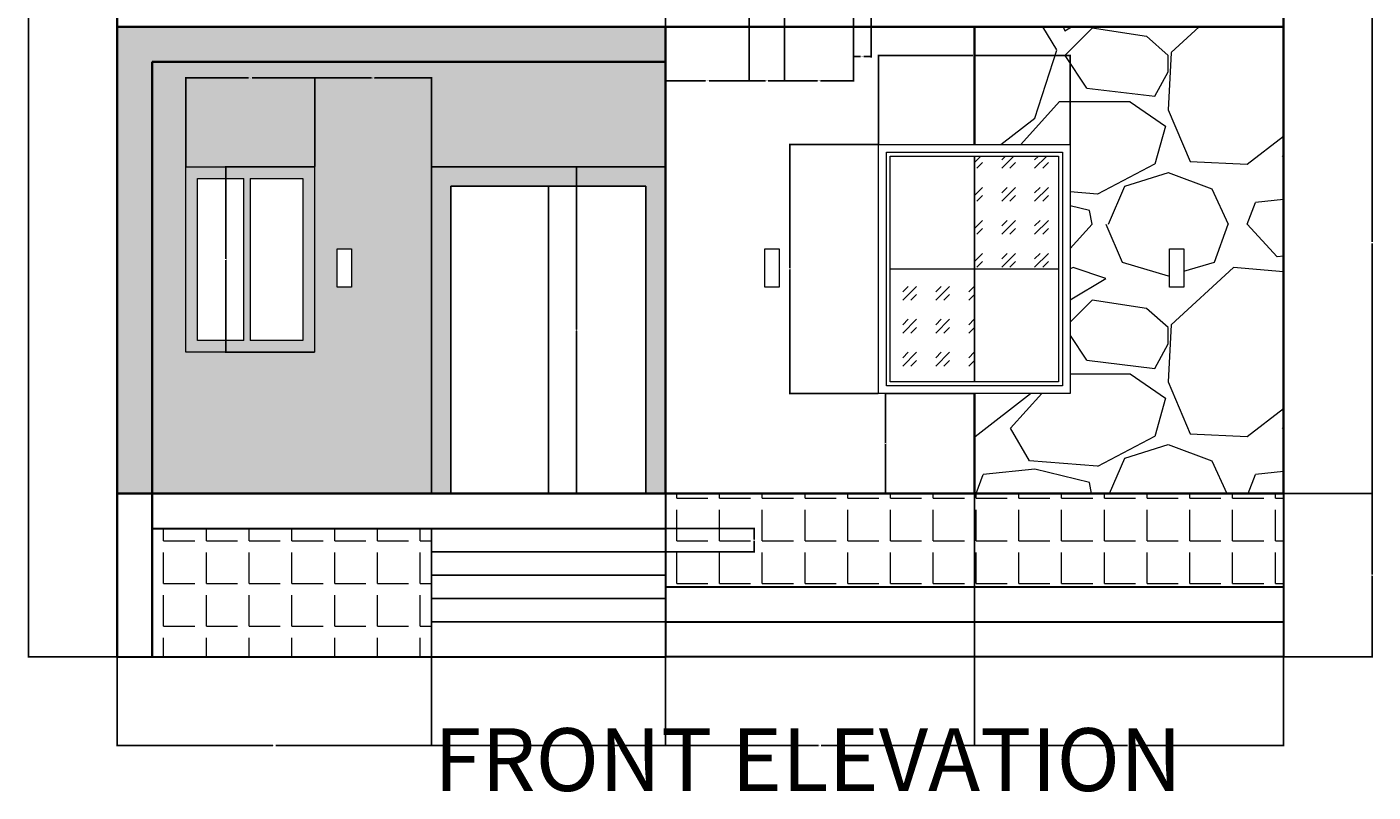
# Model space of a CAD drawing. Units: inches. Extents: x -13 to 333, y -76 to 399.
# Tile 1 of 3: x -13 to 333, y -76 to 121. Entities that reach past the tile are written whole.
import ezdxf

# ---------------------------------------------------------------- set-up
doc = ezdxf.new("R2010")
doc.units = ezdxf.units.IN
doc.header["$MEASUREMENT"] = 0
for name, color, linetype, lineweight in [('A-ANNO-DIMS', 2, 'Continuous', 18), ('A-ANNO-TEXT', 7, 'Continuous', 25), ('A-DOOR', 3, 'Continuous', 25), ('A-ELEV-PATT', 252, 'Continuous', 13), ('A-FLOR', 7, 'Continuous', 35), ('A-FLOR-BASE', 7, 'Continuous', 30), ('A-FLOR-BASE-PATT', 8, 'Continuous', 13), ('A-FLOR-STRS', 7, 'Continuous', 25), ('A-GLAZ', 4, 'Continuous', 18), ('A-GLAZ-PATT', 8, 'Continuous', 13), ('A-WALL', 7, 'Continuous', 35), ('A-WALL-PATT', 252, 'Continuous', 13), ('E-LITE-EXTR', 2, 'Continuous', 18)]:
    doc.layers.add(name, color=color, linetype=linetype, lineweight=lineweight)
doc.styles.get("Standard").update_dxf_attribs({"font": 'arial.ttf'})
doc.dimstyles.get("Standard").update_dxf_attribs({"dimtxt": 0.18, "dimasz": 0.18, "dimexe": 0.18, "dimexo": 0.0625, "dimgap": 0.09, "dimtad": 0, "dimtih": 1, "dimtoh": 1, "dimdec": 4, "dimzin": 0, "dimdsep": 46, "dimtxsty": 'Standard', "dimcen": 0.09, "dimadec": 0, "dimazin": 0, "dimtfac": 1, "dimtdec": 4, "dimtofl": 0, "dimtmove": 0, "dimatfit": 3, "dimfxl": 1, "dimtolj": 1, "dimtzin": 0, "dimarcsym": 0})

# ---------------------------------------------------------------- blocks, each defined once
blk = doc.blocks.new('LIGHT-WALL-SCONCE')
blk.add_lwpolyline([(0, 9.86), (3.7, 9.86), (3.7, 0), (0, 0)], close=True)
blk = doc.blocks.new('*D15')
at = {"layer": 'A-ANNO-DIMS', "color": 0, "lineweight": -2, "transparency": 16777216}
for p, q in [((199.44, 130.11), (199.44, 113.35)), ((203.99, 130.11), (203.99, 113.35)), ((199.62, 113.53), (201.26, 113.53)), ((203.81, 113.53), (202.17, 113.53))]:
    blk.add_line(p, q, dxfattribs=at)
at = {"layer": 'A-ANNO-DIMS', "color": 0, "transparency": 16777216}
for points in [[(199.62, 113.56), (199.62, 113.5), (199.44, 113.53)], [(203.81, 113.56), (203.81, 113.5), (203.99, 113.53)]]:
    blk.add_solid(points, dxfattribs=at)
at = {"layer": 'Defpoints', "color": 0, "transparency": 16777216}
for p in [(199.44, 130.18), (203.99, 130.18), (203.99, 113.53)]:
    blk.add_point(p, dxfattribs=at)
at = {"layer": 'A-ANNO-DIMS', "color": 0, "transparency": 16777216, "insert": (201.71, 113.53), "char_height": 0.18, "attachment_point": 5}
blk.add_mtext('\\A1;5 TYP.', dxfattribs=at)
blk = doc.blocks.new('*D17')
at = {"layer": 'A-ANNO-DIMS', "color": 0, "lineweight": -2, "transparency": 16777216}
for p, q in [((151.01, 375.63), (-12.97, 375.63)), ((-12.79, 375.45), (-12.79, 167.59)), ((-12.79, -40.64), (-12.79, 167.22)), ((10.01, -40.82), (-12.97, -40.82))]:
    blk.add_line(p, q, dxfattribs=at)
at = {"layer": 'A-ANNO-DIMS', "color": 0, "transparency": 16777216}
for points in [[(-12.82, 375.45), (-12.76, 375.45), (-12.79, 375.63)], [(-12.82, -40.64), (-12.76, -40.64), (-12.79, -40.82)]]:
    blk.add_solid(points, dxfattribs=at)
at = {"layer": 'Defpoints', "color": 0, "transparency": 16777216}
for p in [(-12.79, 375.63), (151.07, 375.63), (10.07, -40.82)]:
    blk.add_point(p, dxfattribs=at)
at = {"layer": 'A-ANNO-DIMS', "color": 0, "transparency": 16777216, "insert": (-12.79, 167.4), "char_height": 0.18, "attachment_point": 5}
blk.add_mtext('\\A1;416.46', dxfattribs=at)
blk = doc.blocks.new('*D18')
at = {"layer": 'A-ANNO-DIMS', "color": 0, "lineweight": -2, "transparency": 16777216}
for p, q in [((310.13, 1.18), (333.11, 1.18)), ((332.93, 1), (332.93, -19.64)), ((332.93, -40.64), (332.93, -20)), ((310.13, -40.82), (333.11, -40.82))]:
    blk.add_line(p, q, dxfattribs=at)
at = {"layer": 'A-ANNO-DIMS', "color": 0, "transparency": 16777216}
for points in [[(332.9, 1), (332.96, 1), (332.93, 1.18)], [(332.9, -40.64), (332.96, -40.64), (332.93, -40.82)]]:
    blk.add_solid(points, dxfattribs=at)
at = {"layer": 'Defpoints', "color": 0, "transparency": 16777216}
for p in [(310.07, 1.18), (332.93, 1.18), (310.07, -40.82)]:
    blk.add_point(p, dxfattribs=at)
at = {"layer": 'A-ANNO-DIMS', "color": 0, "transparency": 16777216, "insert": (332.93, -19.82), "char_height": 0.18, "attachment_point": 5}
blk.add_mtext('\\A1;42', dxfattribs=at)
blk = doc.blocks.new('*D19')
at = {"layer": 'A-ANNO-DIMS', "color": 0, "lineweight": -2, "transparency": 16777216}
for p, q in [((310.13, 130.18), (333.11, 130.18)), ((332.93, 130), (332.93, 65.86)), ((332.93, 1.36), (332.93, 65.49)), ((310.13, 1.18), (333.11, 1.18))]:
    blk.add_line(p, q, dxfattribs=at)
at = {"layer": 'A-ANNO-DIMS', "color": 0, "transparency": 16777216}
for points in [[(332.9, 130), (332.96, 130), (332.93, 130.18)], [(332.9, 1.36), (332.96, 1.36), (332.93, 1.18)]]:
    blk.add_solid(points, dxfattribs=at)
at = {"layer": 'Defpoints', "color": 0, "transparency": 16777216}
for p in [(310.07, 130.18), (332.93, 130.18), (310.07, 1.18)]:
    blk.add_point(p, dxfattribs=at)
at = {"layer": 'A-ANNO-DIMS', "color": 0, "transparency": 16777216, "insert": (332.93, 65.68), "char_height": 0.18, "attachment_point": 5}
blk.add_mtext('\\A1;129', dxfattribs=at)
blk = doc.blocks.new('*D22')
at = {"layer": 'A-ANNO-DIMS', "color": 0, "lineweight": -2, "transparency": 16777216}
for p, q in [((10.07, -40.89), (10.07, -63.86)), ((90.91, -40.89), (90.91, -63.86)), ((10.25, -63.68), (50.1, -63.68)), ((90.73, -63.68), (50.88, -63.68))]:
    blk.add_line(p, q, dxfattribs=at)
at = {"layer": 'A-ANNO-DIMS', "color": 0, "transparency": 16777216}
for points in [[(10.25, -63.65), (10.25, -63.71), (10.07, -63.68)], [(90.73, -63.65), (90.73, -63.71), (90.91, -63.68)]]:
    blk.add_solid(points, dxfattribs=at)
at = {"layer": 'Defpoints', "color": 0, "transparency": 16777216}
for p in [(10.07, -40.82), (90.91, -40.82), (90.91, -63.68)]:
    blk.add_point(p, dxfattribs=at)
at = {"layer": 'A-ANNO-DIMS', "color": 0, "transparency": 16777216, "insert": (50.49, -63.68), "char_height": 0.18, "attachment_point": 5}
blk.add_mtext('\\A1;80.84', dxfattribs=at)
blk = doc.blocks.new('*D23')
at = {"layer": 'A-ANNO-DIMS', "color": 0, "lineweight": -2, "transparency": 16777216}
for p, q in [((90.91, -40.89), (90.91, -63.86)), ((151.07, -40.89), (151.07, -63.86)), ((91.09, -63.68), (120.6, -63.68)), ((150.89, -63.68), (121.38, -63.68))]:
    blk.add_line(p, q, dxfattribs=at)
at = {"layer": 'A-ANNO-DIMS', "color": 0, "transparency": 16777216}
for points in [[(91.09, -63.65), (91.09, -63.71), (90.91, -63.68)], [(150.89, -63.65), (150.89, -63.71), (151.07, -63.68)]]:
    blk.add_solid(points, dxfattribs=at)
at = {"layer": 'Defpoints', "color": 0, "transparency": 16777216}
for p in [(90.91, -40.82), (151.07, -40.82), (151.07, -63.68)]:
    blk.add_point(p, dxfattribs=at)
at = {"layer": 'A-ANNO-DIMS', "color": 0, "transparency": 16777216, "insert": (120.99, -63.68), "char_height": 0.18, "attachment_point": 5}
blk.add_mtext('\\A1;60.16', dxfattribs=at)
blk = doc.blocks.new('*D24')
at = {"layer": 'A-ANNO-DIMS', "color": 0, "lineweight": -2, "transparency": 16777216}
for p, q in [((230.57, 1.11), (230.57, -63.86)), ((151.07, -40.89), (151.07, -63.86)), ((151.25, -63.68), (190.5, -63.68)), ((230.39, -63.68), (191.14, -63.68))]:
    blk.add_line(p, q, dxfattribs=at)
at = {"layer": 'A-ANNO-DIMS', "color": 0, "transparency": 16777216}
for points in [[(151.25, -63.65), (151.25, -63.71), (151.07, -63.68)], [(230.39, -63.65), (230.39, -63.71), (230.57, -63.68)]]:
    blk.add_solid(points, dxfattribs=at)
at = {"layer": 'Defpoints', "color": 0, "transparency": 16777216}
for p in [(230.57, 1.18), (151.07, -40.82), (230.57, -63.68)]:
    blk.add_point(p, dxfattribs=at)
at = {"layer": 'A-ANNO-DIMS', "color": 0, "transparency": 16777216, "insert": (190.82, -63.68), "char_height": 0.18, "attachment_point": 5}
blk.add_mtext('\\A1;79.5', dxfattribs=at)
blk = doc.blocks.new('*D25')
at = {"layer": 'A-ANNO-DIMS', "color": 0, "lineweight": -2, "transparency": 16777216}
for p, q in [((230.57, 1.11), (230.57, -63.86)), ((310.07, -40.89), (310.07, -63.86)), ((230.75, -63.68), (270, -63.68)), ((309.89, -63.68), (270.64, -63.68))]:
    blk.add_line(p, q, dxfattribs=at)
at = {"layer": 'A-ANNO-DIMS', "color": 0, "transparency": 16777216}
for points in [[(230.75, -63.65), (230.75, -63.71), (230.57, -63.68)], [(309.89, -63.65), (309.89, -63.71), (310.07, -63.68)]]:
    blk.add_solid(points, dxfattribs=at)
at = {"layer": 'Defpoints', "color": 0, "transparency": 16777216}
for p in [(230.57, 1.18), (310.07, -40.82), (310.07, -63.68)]:
    blk.add_point(p, dxfattribs=at)
at = {"layer": 'A-ANNO-DIMS', "color": 0, "transparency": 16777216, "insert": (270.32, -63.68), "char_height": 0.18, "attachment_point": 5}
blk.add_mtext('\\A1;79.5', dxfattribs=at)
blk = doc.blocks.new('*D26')
at = {"layer": 'A-ANNO-DIMS', "color": 0, "lineweight": -2, "transparency": 16777216}
for p, q in [((27.73, 85.24), (27.73, 108.22)), ((27.91, 108.04), (43.83, 108.04)), ((60.68, 108.04), (44.76, 108.04)), ((60.86, 85.24), (60.86, 108.22))]:
    blk.add_line(p, q, dxfattribs=at)
at = {"layer": 'A-ANNO-DIMS', "color": 0, "transparency": 16777216}
for points in [[(27.91, 108.07), (27.91, 108.01), (27.73, 108.04)], [(60.68, 108.07), (60.68, 108.01), (60.86, 108.04)]]:
    blk.add_solid(points, dxfattribs=at)
at = {"layer": 'Defpoints', "color": 0, "transparency": 16777216}
for p in [(60.86, 108.04), (27.73, 85.18), (60.86, 85.18)]:
    blk.add_point(p, dxfattribs=at)
at = {"layer": 'A-ANNO-DIMS', "color": 0, "transparency": 16777216, "insert": (44.29, 108.04), "char_height": 0.18, "attachment_point": 5}
blk.add_mtext('\\A1;33.124', dxfattribs=at)
blk = doc.blocks.new('*D27')
at = {"layer": 'A-ANNO-DIMS', "color": 0, "lineweight": -2, "transparency": 16777216}
for p, q in [((60.86, 85.24), (60.86, 108.22)), ((61.04, 108.04), (75.49, 108.04)), ((90.73, 108.04), (76.28, 108.04)), ((90.91, 85.24), (90.91, 108.22))]:
    blk.add_line(p, q, dxfattribs=at)
at = {"layer": 'A-ANNO-DIMS', "color": 0, "transparency": 16777216}
for points in [[(61.04, 108.07), (61.04, 108.01), (60.86, 108.04)], [(90.73, 108.07), (90.73, 108.01), (90.91, 108.04)]]:
    blk.add_solid(points, dxfattribs=at)
at = {"layer": 'Defpoints', "color": 0, "transparency": 16777216}
for p in [(90.91, 108.04), (60.86, 85.18), (90.91, 85.18)]:
    blk.add_point(p, dxfattribs=at)
at = {"layer": 'A-ANNO-DIMS', "color": 0, "transparency": 16777216, "insert": (75.88, 108.04), "char_height": 0.18, "attachment_point": 5}
blk.add_mtext('\\A1;30.05', dxfattribs=at)
blk = doc.blocks.new('*D28')
at = {"layer": 'A-ANNO-DIMS', "color": 0, "lineweight": -2, "transparency": 16777216}
for p, q in [((205.93, 91.02), (205.93, 113.99)), ((206.11, 113.81), (230.17, 113.81)), ((255.03, 113.81), (230.97, 113.81)), ((255.21, 91.02), (255.21, 113.99))]:
    blk.add_line(p, q, dxfattribs=at)
at = {"layer": 'A-ANNO-DIMS', "color": 0, "transparency": 16777216}
for points in [[(206.11, 113.84), (206.11, 113.78), (205.93, 113.81)], [(255.03, 113.84), (255.03, 113.78), (255.21, 113.81)]]:
    blk.add_solid(points, dxfattribs=at)
at = {"layer": 'Defpoints', "color": 0, "transparency": 16777216}
for p in [(255.21, 113.81), (205.93, 90.95), (255.21, 90.95)]:
    blk.add_point(p, dxfattribs=at)
at = {"layer": 'A-ANNO-DIMS', "color": 0, "transparency": 16777216, "insert": (230.57, 113.81), "char_height": 0.18, "attachment_point": 5}
blk.add_mtext('\\A1;49.29', dxfattribs=at)
blk = doc.blocks.new('*D29')
at = {"layer": 'A-ANNO-DIMS', "color": 0, "lineweight": -2, "transparency": 16777216}
for p, q in [((60.79, 85.18), (37.82, 85.18)), ((38, 85), (38, 61.55)), ((38, 37.74), (38, 61.19)), ((60.79, 37.56), (37.82, 37.56))]:
    blk.add_line(p, q, dxfattribs=at)
at = {"layer": 'A-ANNO-DIMS', "color": 0, "transparency": 16777216}
for points in [[(37.97, 85), (38.03, 85), (38, 85.18)], [(37.97, 37.74), (38.03, 37.74), (38, 37.56)]]:
    blk.add_solid(points, dxfattribs=at)
at = {"layer": 'Defpoints', "color": 0, "transparency": 16777216}
for p in [(38, 85.18), (60.86, 85.18), (60.86, 37.56)]:
    blk.add_point(p, dxfattribs=at)
at = {"layer": 'A-ANNO-DIMS', "color": 0, "transparency": 16777216, "insert": (38, 61.37), "char_height": 0.18, "attachment_point": 5}
blk.add_mtext('\\A1;47.62', dxfattribs=at)
blk = doc.blocks.new('*D30')
at = {"layer": 'A-ANNO-DIMS', "color": 0, "lineweight": -2, "transparency": 16777216}
for p, q in [((151.01, 85.18), (128.03, 85.18)), ((128.21, 85), (128.21, 43.36)), ((128.21, 1.36), (128.21, 42.99)), ((151.01, 1.18), (128.03, 1.18))]:
    blk.add_line(p, q, dxfattribs=at)
at = {"layer": 'A-ANNO-DIMS', "color": 0, "transparency": 16777216}
for points in [[(128.18, 85), (128.24, 85), (128.21, 85.18)], [(128.18, 1.36), (128.24, 1.36), (128.21, 1.18)]]:
    blk.add_solid(points, dxfattribs=at)
at = {"layer": 'Defpoints', "color": 0, "transparency": 16777216}
for p in [(128.21, 85.18), (151.07, 85.18), (151.07, 1.18)]:
    blk.add_point(p, dxfattribs=at)
at = {"layer": 'A-ANNO-DIMS', "color": 0, "transparency": 16777216, "insert": (128.21, 43.18), "char_height": 0.18, "attachment_point": 5}
blk.add_mtext('\\A1;84', dxfattribs=at)
blk = doc.blocks.new('*D31')
at = {"layer": 'A-ANNO-DIMS', "color": 0, "lineweight": -2, "transparency": 16777216}
for p, q in [((205.86, 90.95), (182.89, 90.95)), ((183.07, 90.77), (183.07, 59.11)), ((183.07, 27.08), (183.07, 58.74)), ((205.86, 26.9), (182.89, 26.9))]:
    blk.add_line(p, q, dxfattribs=at)
at = {"layer": 'A-ANNO-DIMS', "color": 0, "transparency": 16777216}
for points in [[(183.04, 90.77), (183.1, 90.77), (183.07, 90.95)], [(183.04, 27.08), (183.1, 27.08), (183.07, 26.9)]]:
    blk.add_solid(points, dxfattribs=at)
at = {"layer": 'Defpoints', "color": 0, "transparency": 16777216}
for p in [(183.07, 90.95), (205.93, 90.95), (205.93, 26.9)]:
    blk.add_point(p, dxfattribs=at)
at = {"layer": 'A-ANNO-DIMS', "color": 0, "transparency": 16777216, "insert": (183.07, 58.93), "char_height": 0.18, "attachment_point": 5}
blk.add_mtext('\\A1;64.05', dxfattribs=at)
blk = doc.blocks.new('*D32')
at = {"layer": 'A-ANNO-DIMS', "color": 0, "lineweight": -2, "transparency": 16777216}
for p, q in [((230.51, 26.9), (207.53, 26.9)), ((207.71, 26.72), (207.71, 14.22)), ((207.71, 1.36), (207.71, 13.86)), ((230.51, 1.18), (207.53, 1.18))]:
    blk.add_line(p, q, dxfattribs=at)
at = {"layer": 'A-ANNO-DIMS', "color": 0, "transparency": 16777216}
for points in [[(207.68, 26.72), (207.74, 26.72), (207.71, 26.9)], [(207.68, 1.36), (207.74, 1.36), (207.71, 1.18)]]:
    blk.add_solid(points, dxfattribs=at)
at = {"layer": 'Defpoints', "color": 0, "transparency": 16777216}
for p in [(207.71, 26.9), (230.57, 26.9), (230.57, 1.18)]:
    blk.add_point(p, dxfattribs=at)
at = {"layer": 'A-ANNO-DIMS', "color": 0, "transparency": 16777216, "insert": (207.71, 14.04), "char_height": 0.18, "attachment_point": 5}
blk.add_mtext('\\A1;25.723', dxfattribs=at)
blk = doc.blocks.new('*D43')
at = {"layer": 'A-ANNO-DIMS', "color": 0, "lineweight": -2, "transparency": 16777216}
for p, q in [((151.07, 130.11), (151.07, 107.14)), ((172.62, 130.11), (172.62, 107.14)), ((151.25, 107.32), (161.38, 107.32)), ((172.44, 107.32), (162.31, 107.32))]:
    blk.add_line(p, q, dxfattribs=at)
at = {"layer": 'A-ANNO-DIMS', "color": 0, "transparency": 16777216}
for points in [[(151.25, 107.35), (151.25, 107.29), (151.07, 107.32)], [(172.44, 107.35), (172.44, 107.29), (172.62, 107.32)]]:
    blk.add_solid(points, dxfattribs=at)
at = {"layer": 'Defpoints', "color": 0, "transparency": 16777216}
for p in [(151.07, 130.18), (172.62, 130.18), (151.07, 107.32)]:
    blk.add_point(p, dxfattribs=at)
at = {"layer": 'A-ANNO-DIMS', "color": 0, "transparency": 16777216, "insert": (161.84, 107.32), "char_height": 0.18, "attachment_point": 5}
blk.add_mtext('\\A1;21.545', dxfattribs=at)
blk = doc.blocks.new('*D44')
at = {"layer": 'A-ANNO-DIMS', "color": 0, "lineweight": -2, "transparency": 16777216}
for p, q in [((172.62, 130.11), (172.62, 107.14)), ((181.7, 130.11), (181.7, 107.14)), ((172.8, 107.32), (176.83, 107.32)), ((181.52, 107.32), (177.48, 107.32))]:
    blk.add_line(p, q, dxfattribs=at)
at = {"layer": 'A-ANNO-DIMS', "color": 0, "transparency": 16777216}
for points in [[(172.8, 107.35), (172.8, 107.29), (172.62, 107.32)], [(181.52, 107.35), (181.52, 107.29), (181.7, 107.32)]]:
    blk.add_solid(points, dxfattribs=at)
at = {"layer": 'Defpoints', "color": 0, "transparency": 16777216}
for p in [(172.62, 130.18), (181.7, 130.18), (172.62, 107.32)]:
    blk.add_point(p, dxfattribs=at)
at = {"layer": 'A-ANNO-DIMS', "color": 0, "transparency": 16777216, "insert": (177.16, 107.32), "char_height": 0.18, "attachment_point": 5}
blk.add_mtext('\\A1;9.08', dxfattribs=at)
blk = doc.blocks.new('*D45')
at = {"layer": 'A-ANNO-DIMS', "color": 0, "lineweight": -2, "transparency": 16777216}
for p, q in [((181.7, 130.11), (181.7, 107.14)), ((199.44, 130.11), (199.44, 107.14)), ((181.88, 107.32), (190.18, 107.32)), ((199.26, 107.32), (190.96, 107.32))]:
    blk.add_line(p, q, dxfattribs=at)
at = {"layer": 'A-ANNO-DIMS', "color": 0, "transparency": 16777216}
for points in [[(181.88, 107.35), (181.88, 107.29), (181.7, 107.32)], [(199.26, 107.35), (199.26, 107.29), (199.44, 107.32)]]:
    blk.add_solid(points, dxfattribs=at)
at = {"layer": 'Defpoints', "color": 0, "transparency": 16777216}
for p in [(181.7, 130.18), (199.44, 130.18), (181.7, 107.32)]:
    blk.add_point(p, dxfattribs=at)
at = {"layer": 'A-ANNO-DIMS', "color": 0, "transparency": 16777216, "insert": (190.57, 107.32), "char_height": 0.18, "attachment_point": 5}
blk.add_mtext('\\A1;17.75', dxfattribs=at)
blk = doc.blocks.new('*D49')
at = {"layer": 'A-ANNO-DIMS', "color": 0, "lineweight": -2, "transparency": 16777216}
for p, q in [((151.13, -7.82), (174.11, -7.82)), ((173.93, -8), (173.93, -10.64)), ((151.13, -13.82), (174.11, -13.82)), ((173.93, -13.64), (173.93, -11.01))]:
    blk.add_line(p, q, dxfattribs=at)
at = {"layer": 'A-ANNO-DIMS', "color": 0, "transparency": 16777216}
for points in [[(173.9, -8), (173.96, -8), (173.93, -7.82)], [(173.9, -13.64), (173.96, -13.64), (173.93, -13.82)]]:
    blk.add_solid(points, dxfattribs=at)
at = {"layer": 'Defpoints', "color": 0, "transparency": 16777216}
for p in [(151.07, -7.82), (151.07, -13.82), (173.93, -13.82)]:
    blk.add_point(p, dxfattribs=at)
at = {"layer": 'A-ANNO-DIMS', "color": 0, "transparency": 16777216, "insert": (173.93, -10.82), "char_height": 0.18, "attachment_point": 5}
blk.add_mtext('\\A1;6', dxfattribs=at)

msp = doc.modelspace()

# ---------------------------------------------------------------- hatches: boundary and pattern name
at = {"layer": 'A-ELEV-PATT', "transparency": 33554595}
h = msp.add_hatch(color=256, dxfattribs=at)
h.dxf.hatch_style = 1
h.set_gradient(color1=(153, 27, 30), color2=(153, 27, 30))
h.paths.add_polyline_path([(151.0707, 214.1758), (90.9079, 214.1758), (90.9079, 170.2685), (95.9079, 170.2685), (95.9079, 209.1758), (146.0707, 209.1758), (146.0707, 170.2685), (151.0707, 170.2685)])
h.paths.add_polyline_path([(151.0707, 85.1758), (90.9079, 85.1758), (90.9079, 1.1758), (95.9079, 1.1758), (95.9079, 80.1758), (146.0707, 80.1758), (146.0707, 1.1758), (151.0707, 1.1758)])
h.paths.add_polyline_path([(60.8562, 85.1758), (27.7326, 85.1758), (27.7326, 37.5603), (60.8562, 37.5603)])
h.paths.add_polyline_path([(57.8562, 82.1758), (57.8562, 40.5603), (44.2944, 40.5603), (44.2944, 82.1758)], flags=16)
h.paths.add_polyline_path([(42.6571, 82.1758), (42.6571, 40.5603), (30.7326, 40.5603), (30.7326, 82.1758)], flags=16)
at = {"layer": 'A-FLOR-BASE-PATT', "transparency": 33554531}
h = msp.add_hatch(dxfattribs=at)
h.set_pattern_fill('ANGLE', color=256, scale=40)
h.set_pattern_definition([(0, (0, 0), (0, 11), [8, -3]), (90, (0, 0), (-11, 7e-16), [8, -3])])
h.paths.add_polyline_path([(90.9079, -7.8242), (19.0707, -7.8242), (19.0707, -40.8242), (90.9079, -40.8242)])
h.paths.add_polyline_path([(310.0707, 1.1758), (151.0707, 1.1758), (151.0707, -22.8242), (310.0707, -22.8242)])
at = {"layer": 'A-GLAZ-PATT', "transparency": 33554595}
h = msp.add_hatch(dxfattribs=at)
h.set_pattern_fill('GOST_GLASS', color=256)
h.set_pattern_definition([(45, (0, 0), (8.48528, 0), [5, -7]), (45, (2.1213, 0), (8.48528, 0), [2, -10]), (45, (0, 2.1213), (8.48528, 0), [2, -10])])
h.paths.add_polyline_path([(252.2145, 216.9526), (230.5707, 216.9526), (230.5707, 187.9258), (252.2145, 187.9258)])
h.paths.add_polyline_path([(230.5707, 187.9258), (214.7169, 187.9258), (214.7169, 158.899), (230.5707, 158.899)])
h.paths.add_polyline_path([(252.2145, 87.9526), (230.5707, 87.9526), (230.5707, 58.9258), (252.2145, 58.9258)])
h.paths.add_polyline_path([(230.5707, 58.9258), (208.9269, 58.9258), (208.9269, 29.899), (230.5707, 29.899)])
h.paths.add_polyline_path([(252.2145, 342.4077), (230.5707, 342.4077), (230.5707, 313.3809), (252.2145, 313.3809)])
h.paths.add_polyline_path([(230.5707, 313.3809), (208.9269, 313.3809), (208.9269, 295.7236), (230.5707, 295.7236)])
at = {"layer": 'A-WALL-PATT', "transparency": 33554457}
h = msp.add_hatch(color=256, dxfattribs=at)
h.dxf.hatch_style = 1
h.set_gradient(color1=(144, 237, 243), color2=(144, 237, 243), name='HEMISPHERICAL')
h.paths.add_polyline_path([(151.0707, 112.1758), (19.0707, 112.1758), (19.0707, 1.1758), (90.9079, 1.1758), (90.9079, 85.1758), (151.0707, 85.1758)])
h.paths.add_polyline_path([(60.8562, 85.1758), (60.8562, 37.5603), (27.7326, 37.5603), (27.7326, 85.1758)], flags=16)
h.paths.add_polyline_path([(57.8562, 82.1758), (57.8562, 40.5603), (44.2944, 40.5603), (44.2944, 82.1758)], flags=0)
h.paths.add_polyline_path([(70.3288, 64.0624), (70.3288, 54.1998), (66.6308, 54.1998), (66.6308, 64.0624)], flags=16)
h.paths.add_polyline_path([(42.6571, 82.1758), (42.6571, 40.5603), (30.7326, 40.5603), (30.7326, 82.1758)], flags=0)
h.paths.add_polyline_path([(90.9079, 214.1758), (151.0707, 214.1758), (151.0707, 229.1758), (58.0707, 229.1758, 0.41421356), (46.0707, 217.1758), (46.0707, 170.2685), (90.9079, 170.2685)])
h.paths.add_polyline_path([(66.6308, 193.0624), (70.3288, 193.0624), (70.3288, 183.1998), (66.6308, 183.1998)], flags=16)
at = {"layer": 'A-WALL-PATT', "transparency": 33554595}
h = msp.add_hatch(dxfattribs=at)
h.set_pattern_fill('GRAVEL', color=256, scale=70)
h.paths.add_polyline_path([(310.0707, 121.1758), (230.5707, 121.1758), (230.5707, 90.9526), (255.2145, 90.9526), (255.2145, 26.899), (230.5707, 26.899), (230.5707, 1.1758), (310.0707, 1.1758)])
h.paths.add_polyline_path([(280.7936, 64.0624), (284.4916, 64.0624), (284.4916, 54.1998), (280.7936, 54.1998)], flags=16)
h.paths.add_polyline_path([(310.0707, 229.1758), (230.5707, 229.1758), (230.5707, 219.9526), (255.2145, 219.9526), (255.2145, 155.899), (230.5707, 155.899), (230.5707, 130.1758), (310.0707, 130.1758)])
h.paths.add_polyline_path([(280.7936, 183.1998), (280.7936, 193.0624), (284.4916, 193.0624), (284.4916, 183.1998)], flags=16)
h = msp.add_hatch(color=256, dxfattribs=at)
h.dxf.hatch_style = 1
h.set_gradient(color1=(255, 255, 255), name='HEMISPHERICAL')
h.paths.add_polyline_path([(22.0707, 217.1758, -0.11757059), (24.6528, 228.0051), (10.0707, 228.0051), (10.0707, 130.1758), (22.0707, 130.1758)])
h.paths.add_polyline_path([(19.0707, 112.1758), (151.0707, 112.1758), (151.0707, 121.1758), (10.0707, 121.1758), (10.0707, 1.1758), (19.0707, 1.1758)])

# ---------------------------------------------------------------- linework, layer by layer
at = {"layer": 'A-DOOR'}
for p, q in [((146.0707, 80.1758), (95.9079, 80.1758)), ((95.9079, 80.1758), (95.9079, 1.1758)), ((120.9893, 80.1758), (120.9893, 1.1758)), ((146.0707, 1.1758), (146.0707, 80.1758))]:
    msp.add_line(p, q, dxfattribs=at)
msp.add_lwpolyline([(151.0707, 85.1758), (90.9079, 85.1758), (90.9079, 1.1758), (151.0707, 1.1758)], close=True, dxfattribs=at)
at = {"layer": 'A-FLOR'}
for p, q in [((310.0707, 121.1758), (10.0707, 121.1758)), ((10.0707, 1.1758), (151.0707, 1.1758)), ((151.0707, 1.1758), (310.0707, 1.1758))]:
    msp.add_line(p, q, dxfattribs=at)
at = {"layer": 'A-FLOR-BASE'}
for p, q in [((151.0707, 1.1758), (151.0707, -40.8242)), ((310.0707, 1.1758), (310.0707, -40.8242)), ((19.0707, -7.8242), (151.0707, -7.8242)), ((151.0707, -22.8242), (310.0707, -22.8242)), ((151.0707, -31.8242), (310.0707, -31.8242)), ((10.0707, -40.8242), (151.0707, -40.8242)), ((310.0707, -40.8242), (151.0707, -40.8242))]:
    msp.add_line(p, q, dxfattribs=at)
at = {"layer": 'A-FLOR-STRS'}
for p, q in [((90.9079, -7.8242), (90.9079, -40.8242)), ((90.9079, -13.8242), (151.0707, -13.8242)), ((90.9079, -19.8242), (151.0707, -19.8242)), ((90.9079, -25.8242), (151.0707, -25.8242)), ((90.9079, -31.8242), (151.0707, -31.8242))]:
    msp.add_line(p, q, dxfattribs=at)
at = {"layer": 'A-GLAZ'}
for p, q in [((230.5707, 87.9526), (230.5707, 29.899)), ((230.5707, 29.899), (230.5707, 87.9526)), ((208.9269, 58.9258), (252.2145, 58.9258))]:
    msp.add_line(p, q, dxfattribs=at)
for points in [[(205.9269, 90.9526), (255.2145, 90.9526), (255.2145, 26.899), (205.9269, 26.899)], [(207.9269, 88.9526), (253.2145, 88.9526), (253.2145, 28.899), (207.9269, 28.899)], [(208.9269, 87.9526), (252.2145, 87.9526), (252.2145, 29.899), (208.9269, 29.899)], [(27.7326, 85.1758), (60.8562, 85.1758), (60.8562, 37.5603), (27.7326, 37.5603)]]:
    msp.add_lwpolyline(points, close=True, dxfattribs=at)
for points in [[(42.6571, 40.5603), (30.7326, 40.5603), (30.7326, 82.1758), (42.6571, 82.1758)], [(42.6571, 40.5603), (42.6571, 82.1758)], [(44.2944, 82.1758), (44.2944, 40.5603)], [(44.2944, 82.1758), (57.8562, 82.1758), (57.8562, 40.5603), (44.2944, 40.5603)]]:
    msp.add_lwpolyline(points, dxfattribs=at)
at = {"layer": 'A-WALL'}
for p, q in [((10.0707, 121.1758), (10.0707, 241.1758)), ((310.0707, 241.1758), (310.0707, 121.1758)), ((10.0707, 121.1758), (10.0707, -40.8242)), ((151.0707, 121.1758), (151.0707, 1.1758)), ((230.5707, 90.9526), (230.5707, 121.1758)), ((310.0707, 1.1758), (310.0707, 121.1758)), ((19.0707, 112.1758), (19.0707, -40.8242)), ((151.0707, 112.1758), (19.0707, 112.1758)), ((230.5707, 1.1758), (230.5707, 26.899))]:
    msp.add_line(p, q, dxfattribs=at)

# ---------------------------------------------------------------- block references
at = {"layer": 'E-LITE-EXTR'}
for p in [(66.6308, 54.1998), (176.6498, 54.1998), (280.7936, 54.1998)]:
    msp.add_blockref('LIGHT-WALL-SCONCE', p, dxfattribs=at)

# ---------------------------------------------------------------- texts
at = {"layer": 'A-ANNO-TEXT'}
msp.add_text('FRONT ELEVATION', height=16.145751, dxfattribs=at).set_placement((91.5409, -75.3444))

# ---------------------------------------------------------------- dimensions: what is measured, and where the dimension line sits
at = {"layer": 'A-ANNO-DIMS'}
for base, p1, p2, angle, override, picture, middle in [((-12.7893, 375.6309), (10.0707, -40.8242), (151.0707, 375.6309), 90, {"dimdec": 2, "dimlfac": 1, "dimrnd": 0, "dimzin": 0, "dimdsep": 46, "dimlunit": 2}, '*D17', (-12.7893, 167.4033)), ((151.0707, 107.3158), (172.6155, 130.1758), (151.0707, 130.1758), 180, {"dimdec": 3, "dimlfac": 1, "dimrnd": 0, "dimzin": 0, "dimdsep": 46, "dimlunit": 2}, '*D43', (161.8431, 107.3158)), ((172.6155, 107.3158), (181.6962, 130.1758), (172.6155, 130.1758), 180, {"dimdec": 2, "dimlfac": 1, "dimrnd": 0, "dimzin": 0, "dimdsep": 46, "dimlunit": 2}, '*D44', (177.1558, 107.3158)), ((181.6962, 107.3158), (199.4448, 130.1758), (181.6962, 130.1758), 180, {"dimdec": 2, "dimlfac": 1, "dimrnd": 0, "dimzin": 0, "dimdsep": 46, "dimlunit": 2}, '*D45', (190.5705, 107.3158)), ((332.9307, 130.1758), (310.0707, 1.1758), (310.0707, 130.1758), 90, {"dimdec": 0, "dimlfac": 1, "dimrnd": 0, "dimzin": 0, "dimdsep": 46, "dimlunit": 2}, '*D19', (332.9307, 65.6758)), ((183.0669, 90.9526), (205.9269, 26.899), (205.9269, 90.9526), 90, {"dimdec": 2, "dimlfac": 1, "dimrnd": 0, "dimzin": 0, "dimdsep": 46, "dimlunit": 2}, '*D31', (183.0669, 58.9258)), ((37.9962, 85.1758), (60.8562, 37.5603), (60.8562, 85.1758), 90, {"dimdec": 2, "dimlfac": 1, "dimrnd": 0, "dimzin": 0, "dimdsep": 46, "dimlunit": 2}, '*D29', (37.9962, 61.368)), ((128.2107, 85.1758), (151.0707, 1.1758), (151.0707, 85.1758), 90, {"dimdec": 0, "dimlfac": 1, "dimrnd": 0, "dimzin": 0, "dimdsep": 46, "dimlunit": 2}, '*D30', (128.2107, 43.1758)), ((207.7107, 26.899), (230.5707, 1.1758), (230.5707, 26.899), 90, {"dimdec": 3, "dimlfac": 1, "dimrnd": 0, "dimzin": 0, "dimdsep": 46, "dimlunit": 2}, '*D32', (207.7107, 14.0374)), ((332.9307, 1.1758), (310.0707, -40.8242), (310.0707, 1.1758), 90, {"dimdec": 0, "dimlfac": 1, "dimrnd": 0, "dimzin": 0, "dimdsep": 46, "dimlunit": 2}, '*D18', (332.9307, -19.8242)), ((173.9307, -13.8242), (151.0707, -7.8242), (151.0707, -13.8242), 270, {"dimdec": 0, "dimlfac": 1, "dimrnd": 0, "dimzin": 0, "dimdsep": 46, "dimlunit": 2}, '*D49', (173.9307, -10.8242))]:
    dim = msp.add_linear_dim(base=base, p1=p1, p2=p2, angle=angle, dimstyle='Standard', override=override, dxfattribs=at)
    dim.commit()
    dim.dimension.update_dxf_attribs({"geometry": picture, "text_midpoint": middle})
dim = msp.add_linear_dim(base=(203.9852, 113.5258), p1=(199.4448, 130.1758), p2=(203.9852, 130.1758), text='<> TYP.', dimstyle='Standard', override={"dimdec": 0, "dimlfac": 1, "dimrnd": 0, "dimzin": 0, "dimdsep": 46, "dimlunit": 2}, dxfattribs=at)
dim.commit()
dim.dimension.update_dxf_attribs({"geometry": '*D15', "text_midpoint": (201.715, 113.5258)})
for base, p1, p2, override, picture, middle in [((255.2145, 113.8126), (205.9269, 90.9526), (255.2145, 90.9526), {"dimdec": 2, "dimlfac": 1, "dimrnd": 0, "dimzin": 0, "dimdsep": 46, "dimlunit": 2}, '*D28', (230.5707, 113.8126)), ((60.8562, 108.0358), (27.7326, 85.1758), (60.8562, 85.1758), {"dimdec": 3, "dimlfac": 1, "dimrnd": 0, "dimzin": 0, "dimdsep": 46, "dimlunit": 2}, '*D26', (44.2944, 108.0358)), ((90.9079, 108.0358), (60.8562, 85.1758), (90.9079, 85.1758), {"dimdec": 2, "dimlfac": 1, "dimrnd": 0, "dimzin": 0, "dimdsep": 46, "dimlunit": 2}, '*D27', (75.882, 108.0358)), ((230.5707, -63.6842), (151.0707, -40.8242), (230.5707, 1.1758), {"dimdec": 1, "dimlfac": 1, "dimrnd": 0, "dimzin": 0, "dimdsep": 46, "dimlunit": 2}, '*D24', (190.8207, -63.6842)), ((310.0707, -63.6842), (230.5707, 1.1758), (310.0707, -40.8242), {"dimdec": 1, "dimlfac": 1, "dimrnd": 0, "dimzin": 0, "dimdsep": 46, "dimlunit": 2}, '*D25', (270.3207, -63.6842)), ((90.9079, -63.6842), (10.0707, -40.8242), (90.9079, -40.8242), {"dimdec": 2, "dimlfac": 1, "dimrnd": 0, "dimzin": 0, "dimdsep": 46, "dimlunit": 2}, '*D22', (50.4893, -63.6842)), ((151.0707, -63.6842), (90.9079, -40.8242), (151.0707, -40.8242), {"dimdec": 2, "dimlfac": 1, "dimrnd": 0, "dimzin": 0, "dimdsep": 46, "dimlunit": 2}, '*D23', (120.9893, -63.6842))]:
    dim = msp.add_linear_dim(base=base, p1=p1, p2=p2, dimstyle='Standard', override=override, dxfattribs=at)
    dim.commit()
    dim.dimension.update_dxf_attribs({"geometry": picture, "text_midpoint": middle})

doc.saveas('drawing.dxf')
